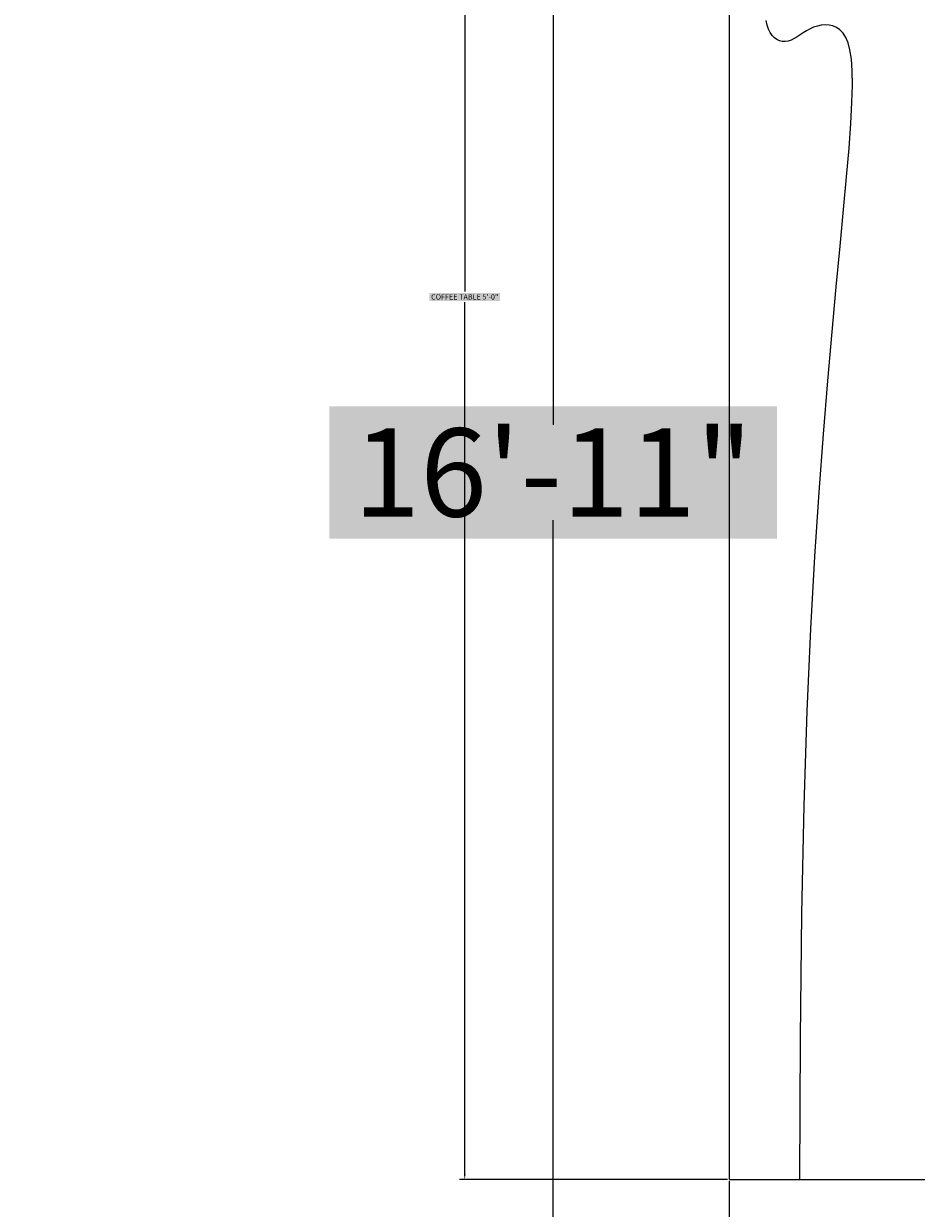
# Model space of a CAD drawing. Units: inches. Extents: x -301 to 715, y -607 to 364.
# Tile 106 of 141: x 16 to 46, y 67 to 107. Entities that reach past the tile are written whole.
import ezdxf

# ---------------------------------------------------------------- set-up
doc = ezdxf.new("R2010")
doc.units = ezdxf.units.IN
doc.header["$MEASUREMENT"] = 0
doc.layers.add('A-ANNO-DIMS', color=2, linetype='Continuous', lineweight=18)
doc.layers.add('A-FURN', color=8, linetype='Continuous', lineweight=18)
doc.styles.get("Standard").update_dxf_attribs({"font": 'arial.ttf'})
doc.dimstyles.get("Standard").update_dxf_attribs({"dimtxt": 0.18, "dimasz": 0.18, "dimexe": 0.18, "dimexo": 0.0625, "dimgap": 0.09, "dimtad": 0, "dimtih": 1, "dimtoh": 1, "dimdec": 1, "dimzin": 0, "dimdsep": 46, "dimlunit": 4, "dimtxsty": 'Standard', "dimcen": 0.09, "dimclrd": 3, "dimclre": 4, "dimclrt": 6, "dimadec": 0, "dimazin": 0, "dimtfac": 1, "dimtdec": 1, "dimtofl": 0, "dimtmove": 0, "dimatfit": 3, "dimfxl": 1, "dimtfill": 2, "dimtfillclr": 51, "dimtolj": 1, "dimtzin": 0, "dimarcsym": 0})

# ---------------------------------------------------------------- blocks, each defined once
blk = doc.blocks.new('Table - Rectangular Woodgrain 60 x 30 in.')
for p, q in [((0, 0), (0, -30)), ((60, 0), (0, 0))]:
    blk.add_line(p, q)
blk.add_lwpolyline([(0, -2.4), (4.8155, -2.418), (9.0302, -2.4688), (12.709, -2.5477), (15.9167, -2.65), (18.7181, -2.7711), (21.1781, -2.9063), (23.3616, -3.0508), (25.3333, -3.2), (27.1477, -3.3495), (28.8172, -3.4958), (30.3437, -3.636), (31.7291, -3.7667), (32.9756, -3.8849), (34.0849, -3.9875), (35.059, -4.0714), (35.9, -4.1334), (36.6114, -4.1711), (37.2041, -4.1854), (37.6906, -4.1779), (38.0833, -4.15), (38.3948, -4.1034), (38.6375, -4.0396), (38.8239, -3.9602), (38.9666, -3.8667), (39.0764, -3.7608), (39.1573, -3.6448), (39.2116, -3.521), (39.2416, -3.3917), (39.2498, -3.2593), (39.2385, -3.1261), (39.21, -2.9944), (39.1666, -2.8667), (39.111, -2.7447), (39.0468, -2.6281), (38.978, -2.5163), (38.9083, -2.4083), (38.8418, -2.3035), (38.7823, -2.201), (38.7337, -2.1001), (38.7, -2), (38.6844, -1.9003), (38.6875, -1.8021), (38.7094, -1.707), (38.75, -1.6167), (38.8094, -1.5326), (38.8875, -1.4563), (38.9844, -1.3893), (39.1, -1.3333), (39.2351, -1.2896), (39.3937, -1.2583)])
blk = doc.blocks.new('*D49')
at = {"layer": 'A-ANNO-DIMS', "color": 0, "lineweight": -2, "transparency": 16777216}
for p, q in [((15.959, 193.182), (34.084, 193.182)), ((33.904, 188.182), (33.904, 93.304)), ((33.904, -4.818), (33.904, 90.061)), ((21.959, -9.818), (34.084, -9.818))]:
    blk.add_line(p, q, dxfattribs=at)
at = {"layer": 'A-ANNO-DIMS', "color": 0, "transparency": 16777216}
for points in [[(33.071, 188.182), (34.737, 188.182), (33.904, 193.182)], [(33.071, -4.818), (34.737, -4.818), (33.904, -9.818)]]:
    blk.add_solid(points, dxfattribs=at)
at = {"layer": 'Defpoints', "color": 0, "transparency": 16777216}
for p in [(15.897, 193.182), (33.904, 193.182), (21.897, -9.818)]:
    blk.add_point(p, dxfattribs=at)
at = {"layer": 'A-ANNO-DIMS', "color": 0, "transparency": 16777216, "insert": (33.904, 91.682), "char_height": 3, "attachment_point": 5, "bg_fill": 1, "box_fill_scale": 1.25, "bg_fill_color": 51, "bg_fill_transparency": 0}
blk.add_mtext('\\A1;16\'-11"', dxfattribs=at)
blk = doc.blocks.new('*D130')
at = {"layer": 'A-ANNO-DIMS', "color": 4, "lineweight": -2, "transparency": 16777216}
for p, q in [((39.835, 127.651), (30.717, 127.651)), ((39.835, 67.651), (30.717, 67.651))]:
    blk.add_line(p, q, dxfattribs=at)
at = {"layer": 'A-ANNO-DIMS', "color": 3, "lineweight": -2, "transparency": 16777216}
for p, q in [((30.897, 127.471), (30.897, 97.834)), ((30.897, 67.831), (30.897, 97.467))]:
    blk.add_line(p, q, dxfattribs=at)
at = {"layer": 'A-ANNO-DIMS', "color": 3, "transparency": 16777216}
for points in [[(30.867, 127.471), (30.927, 127.471), (30.897, 127.651)], [(30.867, 67.831), (30.927, 67.831), (30.897, 67.651)]]:
    blk.add_solid(points, dxfattribs=at)
at = {"layer": 'Defpoints', "color": 0, "transparency": 16777216}
for p in [(30.897, 127.651), (39.897, 127.651), (39.897, 67.651)]:
    blk.add_point(p, dxfattribs=at)
at = {"layer": 'A-ANNO-DIMS', "color": 6, "transparency": 16777216, "insert": (30.897, 97.651), "char_height": 0.18, "attachment_point": 5, "bg_fill": 1, "box_fill_scale": 1.25, "bg_fill_color": 51, "bg_fill_transparency": 0}
blk.add_mtext('\\A1;COFFEE TABLE 5\'-0"', dxfattribs=at)
blk = doc.blocks.new('*D131')
at = {"layer": 'A-ANNO-DIMS', "color": 4, "lineweight": -2, "transparency": 16777216}
for p, q in [((39.897, 67.588), (39.897, 58.471)), ((69.897, 67.588), (69.897, 58.471))]:
    blk.add_line(p, q, dxfattribs=at)
at = {"layer": 'A-ANNO-DIMS', "color": 3, "lineweight": -2, "transparency": 16777216}
for p, q in [((40.077, 58.651), (54.566, 58.651)), ((69.717, 58.651), (55.228, 58.651))]:
    blk.add_line(p, q, dxfattribs=at)
at = {"layer": 'A-ANNO-DIMS', "color": 3, "transparency": 16777216}
for points in [[(40.077, 58.681), (40.077, 58.621), (39.897, 58.651)], [(69.717, 58.681), (69.717, 58.621), (69.897, 58.651)]]:
    blk.add_solid(points, dxfattribs=at)
at = {"layer": 'Defpoints', "color": 0, "transparency": 16777216}
for p in [(39.897, 67.651), (69.897, 67.651), (39.897, 58.651)]:
    blk.add_point(p, dxfattribs=at)
at = {"layer": 'A-ANNO-DIMS', "color": 6, "transparency": 16777216, "insert": (54.897, 58.651), "char_height": 0.18, "attachment_point": 5, "bg_fill": 1, "box_fill_scale": 1.25, "bg_fill_color": 51, "bg_fill_transparency": 0}
blk.add_mtext('\\A1;2\'-6"', dxfattribs=at)

msp = doc.modelspace()

# ---------------------------------------------------------------- block references
at = {"layer": 'A-FURN', "rotation": 90}
msp.add_blockref('Table - Rectangular Woodgrain 60 x 30 in.', (39.897, 67.651), dxfattribs=at)

# ---------------------------------------------------------------- dimensions: what is measured, and where the dimension line sits
at = {"layer": 'A-ANNO-DIMS'}
for base, p1, p2, angle, override, picture, middle in [((33.904, 193.182), (21.897, -9.818), (15.897, 193.182), 90, {"dimtxt": 3, "dimasz": 5, "dimclrd": 0, "dimclre": 0, "dimclrt": 0}, '*D49', (33.904, 91.682)), ((39.897, 58.651), (69.897, 67.651), (39.897, 67.651), 180, {"dimdec": 1, "dimlfac": 1, "dimrnd": 0, "dimzin": 1, "dimdsep": 46, "dimlunit": 4, "dimfrac": 2}, '*D131', (54.897, 58.651))]:
    dim = msp.add_linear_dim(base=base, p1=p1, p2=p2, angle=angle, dimstyle='Standard', override=override, dxfattribs=at)
    dim.commit()
    dim.dimension.update_dxf_attribs({"geometry": picture, "text_midpoint": middle})
dim = msp.add_linear_dim(base=(30.897, 127.651), p1=(39.897, 67.651), p2=(39.897, 127.651), angle=90, text='COFFEE TABLE <>', dimstyle='Standard', override={"dimdec": 1, "dimlfac": 1, "dimrnd": 0, "dimzin": 1, "dimdsep": 46, "dimlunit": 4, "dimfrac": 2}, dxfattribs=at)
dim.commit()
dim.dimension.update_dxf_attribs({"geometry": '*D130', "text_midpoint": (30.897, 97.651)})

doc.saveas('drawing.dxf')
